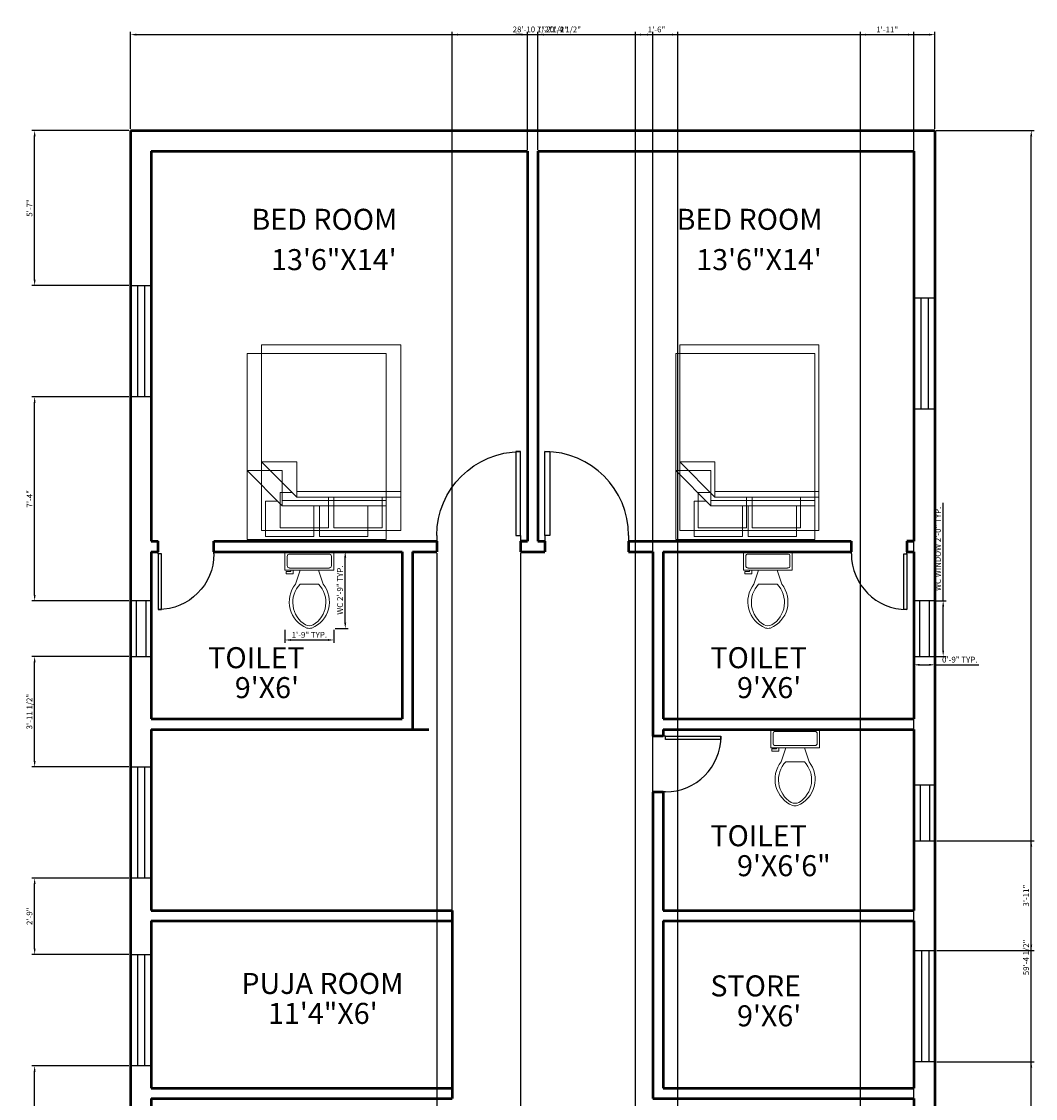
# Model space of a CAD drawing. Units: inches. Extents: x 2691 to 8091, y 3734 to 9067.
# Tile 4 of 5: x 2691 to 3127, y 4181 to 4645. Entities that reach past the tile are written whole.
import ezdxf

# ---------------------------------------------------------------- set-up
doc = ezdxf.new("R2010")
doc.units = ezdxf.units.IN
doc.layers.get('0').update_dxf_attribs({"color": 80})
for name, color, linetype, lineweight in [('A-ANNO-DIMS', 2, 'Continuous', 18), ('A-AREA-IDEN', 7, 'Continuous', 18), ('A-FLOR-FIXT', 9, 'Continuous', 18), ('A-FURN', 8, 'Continuous', 18), ('A-WALL', 50, 'Continuous', 50), ('doors', 10, 'Continuous', 25), ('window', 4, 'Continuous', 25)]:
    doc.layers.add(name, color=color, linetype=linetype, lineweight=lineweight)
doc.styles.get("Standard").update_dxf_attribs({"font": 'arial.ttf'})
doc.dimstyles.new('ISO-25', dxfattribs={"dimtxt": 2.5, "dimasz": 2.5, "dimexe": 1.25, "dimexo": 0.625, "dimtad": 1, "dimdec": 1, "dimlunit": 3, "dimtxsty": 'Standard', "dimcen": 2.5, "dimadec": 0, "dimazin": 0, "dimtfac": 1, "dimtdec": 1, "dimtmove": 0, "dimatfit": 3, "dimfxl": 1, "dimarcsym": 0})

# ---------------------------------------------------------------- blocks, each defined once
blk = doc.blocks.new('Bed - Queen')
for p, q in [((0, -80.00003), (0, 0)), ((0, 0), (59.99999, 0)), ((59.99999, 0), (59.99999, -80.00003)), ((7.99999, -1.2), (28.79998, -1.2)), ((7.99999, -14.4), (7.99999, -1.2)), ((28.79998, -1.2), (28.79998, -14.4)), ((31.19999, -1.2), (51.99999, -1.2)), ((31.19999, -14.4), (31.19999, -1.2)), ((51.99999, -1.2), (51.99999, -16.4)), ((0, -14.4), (44.8, -14.4)), ((44.8, -16.8), (0, -16.8)), ((59.99999, -29.6), (44.8, -14.4)), ((44.8, -14.4), (44.8, -29.6)), ((51.99999, -16.4), (46.79936, -16.4)), ((44.8, -29.6), (59.99999, -29.6)), ((59.99999, -80.00003), (0, -80.00003))]:
    blk.add_line(p, q)
blk = doc.blocks.new('Toilet - top')
for p, q in [((9.5, -6), (9.5, -2)), ((-10, -8.5), (-8, -8.5)), ((-10, -9.5), (-10, -8.5)), ((-8, -8.5), (-8, -8)), ((-7, -8), (-7, -9.5)), ((-4, -8), (-6, -14)), ((4, -8), (6, -14)), ((-7, -9.5), (-10, -9.5)), ((4, -14), (-4, -14))]:
    blk.add_line(p, q)
blk.add_lwpolyline([(10.5, -8), (10.5, 0), (-10.5, 0), (-10.5, -8)], close=True)
for points in [[(-9.5, -2), (-9.5, -6)], [(8.5, -1), (-8.5, -1)], [(-8.5, -7), (8.5, -7)]]:
    blk.add_lwpolyline(points)
for centre, radius, start, end in [((-8.62, -1.88), 0.884, 81.8699, 188.1301), ((8.62, -1.88), 0.884, 351.8699, 98.1301), ((-8.62, -6.12), 0.884, 171.8699, 278.1301), ((8.62, -6.12), 0.884, 261.8699, 8.1301), ((3.52, -21.58), 12.17, 141.4691, 247.9714), ((4.2, -21.82), 11.33, 136.3677, 238.9468), ((-3.52, -21.58), 12.17, 292.0284, 38.5307), ((-4.2, -21.82), 11.33, 301.053, 43.6321), ((0, -27.88), 4, 245.7318, 294.2682), ((0, -29), 4, 254.8605, 285.1395)]:
    blk.add_arc(centre, radius, start, end)
blk = doc.blocks.new('Dining Set - 36 x 72 in')
at = {"layer": 'window'}
for p, q in [((418.4, 887.02), (466.4, 887.02)), ((418.4, 883.92), (466.4, 883.92))]:
    blk.add_line(p, q, dxfattribs=at)
blk.add_lwpolyline([(418.4, 881.14), (418.4, 890.14), (466.4, 890.14), (466.4, 881.14)], close=True, dxfattribs=at)
blk = doc.blocks.new('new block')
at = {"layer": 'window'}
for p, q in [((-15.79, 35.68), (-15.79, 11.68)), ((-11.65, 35.68), (-11.65, 11.68))]:
    blk.add_line(p, q, dxfattribs=at)
blk.add_lwpolyline([(-9.22, 35.68), (-18.22, 35.68), (-18.22, 11.68), (-9.22, 11.68)], close=True, dxfattribs=at)
blk = doc.blocks.new('*U13')
for p, q in [((0, 0), (0, -100)), ((750, 0), (750, -100))]:
    blk.add_line(p, q)
blk.add_lwpolyline([(0, 0), (0, 750), (43.75, 750), (43.75, 0)], close=True)
blk.add_arc((0, 0), 750, 0, 90)
blk = doc.blocks.new('*D23')
at = {"layer": 'A-ANNO-DIMS', "color": 0, "lineweight": -2, "transparency": 16777216}
for p, q in [((3087.56, 4395.22), (3087.56, 4437.39)), ((3084.58, 4395.22), (3088.81, 4395.22)), ((3087.56, 4373.72), (3087.56, 4392.72)), ((3084.58, 4371.22), (3088.81, 4371.22))]:
    blk.add_line(p, q, dxfattribs=at)
at = {"layer": 'A-ANNO-DIMS', "color": 0, "transparency": 16777216}
for points in [[(3087.14, 4392.72), (3087.98, 4392.72), (3087.56, 4395.22)], [(3087.14, 4373.72), (3087.98, 4373.72), (3087.56, 4371.22)]]:
    blk.add_solid(points, dxfattribs=at)
at = {"layer": 'Defpoints', "color": 0, "transparency": 16777216}
for p in [(3083.96, 4395.22), (3087.56, 4395.22), (3083.96, 4371.22)]:
    blk.add_point(p, dxfattribs=at)
at = {"layer": 'A-ANNO-DIMS', "color": 0, "transparency": 16777216, "insert": (3085.64, 4417.56), "char_height": 2.5, "attachment_point": 5, "rotation": 90}
blk.add_mtext('WC WINDOW 2\'-0" TYP.', dxfattribs=at)
blk = doc.blocks.new('*D24')
at = {"layer": 'A-ANNO-DIMS', "color": 0, "lineweight": -2, "transparency": 16777216}
for p, q in [((3074.96, 4370.59), (3074.96, 4366.37)), ((3083.96, 4370.59), (3083.96, 4366.37)), ((3077.46, 4367.62), (3081.46, 4367.62)), ((3083.96, 4367.62), (3102.95, 4367.62))]:
    blk.add_line(p, q, dxfattribs=at)
at = {"layer": 'A-ANNO-DIMS', "color": 0, "transparency": 16777216}
for points in [[(3077.46, 4368.04), (3077.46, 4367.2), (3074.96, 4367.62)], [(3081.46, 4368.04), (3081.46, 4367.2), (3083.96, 4367.62)]]:
    blk.add_solid(points, dxfattribs=at)
at = {"layer": 'Defpoints', "color": 0, "transparency": 16777216}
for p in [(3074.96, 4371.22), (3083.96, 4371.22), (3083.96, 4367.62)]:
    blk.add_point(p, dxfattribs=at)
at = {"layer": 'A-ANNO-DIMS', "color": 0, "transparency": 16777216, "insert": (3094.7, 4369.52), "char_height": 2.5, "attachment_point": 5}
blk.add_mtext('0\'-9" TYP.', dxfattribs=at)
blk = doc.blocks.new('*D31')
at = {"layer": 'A-ANNO-DIMS', "color": 0, "lineweight": -2, "transparency": 16777216}
for p, q in [((2825.66, 4416.32), (2831.24, 4416.32)), ((2829.99, 4385.77), (2829.99, 4413.82)), ((2825.66, 4383.27), (2831.24, 4383.27))]:
    blk.add_line(p, q, dxfattribs=at)
at = {"layer": 'A-ANNO-DIMS', "color": 0, "transparency": 16777216}
for points in [[(2829.57, 4413.82), (2830.41, 4413.82), (2829.99, 4416.32)], [(2829.57, 4385.77), (2830.41, 4385.77), (2829.99, 4383.27)]]:
    blk.add_solid(points, dxfattribs=at)
at = {"layer": 'Defpoints', "color": 0, "transparency": 16777216}
for p in [(2825.03, 4416.32), (2829.99, 4416.32), (2825.03, 4383.27)]:
    blk.add_point(p, dxfattribs=at)
at = {"layer": 'A-ANNO-DIMS', "color": 0, "transparency": 16777216, "insert": (2828.07, 4399.8), "char_height": 2.5, "attachment_point": 5, "rotation": 90}
blk.add_mtext('WC 2\'-9" TYP.', dxfattribs=at)
blk = doc.blocks.new('*D32')
at = {"layer": 'A-ANNO-DIMS', "color": 0, "lineweight": -2, "transparency": 16777216}
for p, q in [((2804.03, 4382.65), (2804.03, 4377.07)), ((2825.03, 4382.65), (2825.03, 4377.07)), ((2806.53, 4378.32), (2822.53, 4378.32))]:
    blk.add_line(p, q, dxfattribs=at)
at = {"layer": 'A-ANNO-DIMS', "color": 0, "transparency": 16777216}
for points in [[(2806.53, 4378.73), (2806.53, 4377.9), (2804.03, 4378.32)], [(2822.53, 4378.73), (2822.53, 4377.9), (2825.03, 4378.32)]]:
    blk.add_solid(points, dxfattribs=at)
at = {"layer": 'Defpoints', "color": 0, "transparency": 16777216}
for p in [(2804.03, 4383.27), (2825.03, 4383.27), (2825.03, 4378.32)]:
    blk.add_point(p, dxfattribs=at)
at = {"layer": 'A-ANNO-DIMS', "color": 0, "transparency": 16777216, "insert": (2814.53, 4380.22), "char_height": 2.5, "attachment_point": 5}
blk.add_mtext('1\'-9" TYP.', dxfattribs=at)
blk = doc.blocks.new('*D45')
at = {"layer": 'A-ANNO-DIMS', "color": 0, "lineweight": -2, "transparency": 16777216}
for p, q in [((2736.83, 4597.82), (2694.95, 4597.82)), ((2696.2, 4533.51), (2696.2, 4595.32)), ((2736.83, 4531.01), (2694.95, 4531.01))]:
    blk.add_line(p, q, dxfattribs=at)
at = {"layer": 'A-ANNO-DIMS', "color": 0, "transparency": 16777216}
for points in [[(2695.79, 4595.32), (2696.62, 4595.32), (2696.2, 4597.82)], [(2695.79, 4533.51), (2696.62, 4533.51), (2696.2, 4531.01)]]:
    blk.add_solid(points, dxfattribs=at)
at = {"layer": 'Defpoints', "color": 0, "transparency": 16777216}
for p in [(2696.2, 4597.82), (2737.46, 4597.82), (2737.46, 4531.01)]:
    blk.add_point(p, dxfattribs=at)
at = {"layer": 'A-ANNO-DIMS', "color": 0, "transparency": 16777216, "insert": (2694.31, 4564.41), "char_height": 2.5, "attachment_point": 5, "rotation": 90}
blk.add_mtext('5\'-7"', dxfattribs=at)
blk = doc.blocks.new('*D46')
at = {"layer": 'A-ANNO-DIMS', "color": 0, "lineweight": -2, "transparency": 16777216}
for p, q in [((2736.83, 4483.01), (2694.95, 4483.01)), ((2696.2, 4397.72), (2696.2, 4480.51)), ((2736.83, 4395.22), (2694.95, 4395.22))]:
    blk.add_line(p, q, dxfattribs=at)
at = {"layer": 'A-ANNO-DIMS', "color": 0, "transparency": 16777216}
for points in [[(2695.79, 4480.51), (2696.62, 4480.51), (2696.2, 4483.01)], [(2695.79, 4397.72), (2696.62, 4397.72), (2696.2, 4395.22)]]:
    blk.add_solid(points, dxfattribs=at)
at = {"layer": 'Defpoints', "color": 0, "transparency": 16777216}
for p in [(2696.2, 4483.01), (2737.46, 4483.01), (2737.45, 4395.22)]:
    blk.add_point(p, dxfattribs=at)
at = {"layer": 'A-ANNO-DIMS', "color": 0, "transparency": 16777216, "insert": (2694.33, 4439.11), "char_height": 2.5, "attachment_point": 5, "rotation": 90}
blk.add_mtext('7\'-4"', dxfattribs=at)
blk = doc.blocks.new('*D47')
at = {"layer": 'A-ANNO-DIMS', "color": 0, "lineweight": -2, "transparency": 16777216}
for p, q in [((2736.83, 4371.22), (2694.95, 4371.22)), ((2696.2, 4326.17), (2696.2, 4368.72)), ((2736.83, 4323.67), (2694.95, 4323.67))]:
    blk.add_line(p, q, dxfattribs=at)
at = {"layer": 'A-ANNO-DIMS', "color": 0, "transparency": 16777216}
for points in [[(2695.79, 4368.72), (2696.62, 4368.72), (2696.2, 4371.22)], [(2695.79, 4326.17), (2696.62, 4326.17), (2696.2, 4323.67)]]:
    blk.add_solid(points, dxfattribs=at)
at = {"layer": 'Defpoints', "color": 0, "transparency": 16777216}
for p in [(2696.2, 4371.22), (2737.45, 4371.22), (2737.46, 4323.67)]:
    blk.add_point(p, dxfattribs=at)
at = {"layer": 'A-ANNO-DIMS', "color": 0, "transparency": 16777216, "insert": (2694.28, 4347.45), "char_height": 2.5, "attachment_point": 5, "rotation": 90}
blk.add_mtext('3\'-11 1/2"', dxfattribs=at)
blk = doc.blocks.new('*D48')
at = {"layer": 'A-ANNO-DIMS', "color": 0, "lineweight": -2, "transparency": 16777216}
for p, q in [((2736.83, 4275.67), (2694.95, 4275.67)), ((2696.2, 4245.39), (2696.2, 4273.17)), ((2736.83, 4242.89), (2694.95, 4242.89))]:
    blk.add_line(p, q, dxfattribs=at)
at = {"layer": 'A-ANNO-DIMS', "color": 0, "transparency": 16777216}
for points in [[(2695.79, 4273.17), (2696.62, 4273.17), (2696.2, 4275.67)], [(2695.79, 4245.39), (2696.62, 4245.39), (2696.2, 4242.89)]]:
    blk.add_solid(points, dxfattribs=at)
at = {"layer": 'Defpoints', "color": 0, "transparency": 16777216}
for p in [(2696.2, 4275.67), (2737.46, 4275.67), (2737.46, 4242.89)]:
    blk.add_point(p, dxfattribs=at)
at = {"layer": 'A-ANNO-DIMS', "color": 0, "transparency": 16777216, "insert": (2694.3, 4259.28), "char_height": 2.5, "attachment_point": 5, "rotation": 90}
blk.add_mtext('2\'-9"', dxfattribs=at)
blk = doc.blocks.new('*D49')
at = {"layer": 'A-ANNO-DIMS', "color": 0, "lineweight": -2, "transparency": 16777216}
for p, q in [((2736.83, 4194.89), (2694.95, 4194.89)), ((2696.2, 4114.35), (2696.2, 4192.39)), ((2736.83, 4111.85), (2694.95, 4111.85))]:
    blk.add_line(p, q, dxfattribs=at)
at = {"layer": 'A-ANNO-DIMS', "color": 0, "transparency": 16777216}
for points in [[(2695.79, 4192.39), (2696.62, 4192.39), (2696.2, 4194.89)], [(2695.79, 4114.35), (2696.62, 4114.35), (2696.2, 4111.85)]]:
    blk.add_solid(points, dxfattribs=at)
at = {"layer": 'Defpoints', "color": 0, "transparency": 16777216}
for p in [(2696.2, 4194.89), (2737.46, 4194.89), (2737.46, 4111.85)]:
    blk.add_point(p, dxfattribs=at)
at = {"layer": 'A-ANNO-DIMS', "color": 0, "transparency": 16777216, "insert": (2694.3, 4153.37), "char_height": 2.5, "attachment_point": 5, "rotation": 90}
blk.add_mtext('6\'-11"', dxfattribs=at)
blk = doc.blocks.new('*D54')
at = {"layer": 'A-ANNO-DIMS', "color": 0, "lineweight": -2, "transparency": 16777216}
for p, q in [((3084.79, 4291.79), (3126.76, 4291.79)), ((3125.51, 4247.07), (3125.51, 4289.29)), ((3084.88, 4244.57), (3126.76, 4244.57))]:
    blk.add_line(p, q, dxfattribs=at)
at = {"layer": 'A-ANNO-DIMS', "color": 0, "transparency": 16777216}
for points in [[(3125.09, 4289.29), (3125.92, 4289.29), (3125.51, 4291.79)], [(3125.09, 4247.07), (3125.92, 4247.07), (3125.51, 4244.57)]]:
    blk.add_solid(points, dxfattribs=at)
at = {"layer": 'Defpoints', "color": 0, "transparency": 16777216}
for p in [(3084.16, 4291.79), (3125.51, 4291.79), (3084.26, 4244.57)]:
    blk.add_point(p, dxfattribs=at)
at = {"layer": 'A-ANNO-DIMS', "color": 0, "transparency": 16777216, "insert": (3123.6, 4268.18), "char_height": 2.5, "attachment_point": 5, "rotation": 90}
blk.add_mtext('3\'-11"', dxfattribs=at)
blk = doc.blocks.new('*D55')
at = {"layer": 'A-ANNO-DIMS', "color": 0, "lineweight": -2, "transparency": 16777216}
for p, q in [((3084.88, 4196.57), (3126.76, 4196.57)), ((3125.51, 4126.91), (3125.51, 4194.07)), ((3084.58, 4124.41), (3126.76, 4124.41))]:
    blk.add_line(p, q, dxfattribs=at)
at = {"layer": 'A-ANNO-DIMS', "color": 0, "transparency": 16777216}
for points in [[(3125.09, 4194.07), (3125.92, 4194.07), (3125.51, 4196.57)], [(3125.09, 4126.91), (3125.92, 4126.91), (3125.51, 4124.41)]]:
    blk.add_solid(points, dxfattribs=at)
at = {"layer": 'Defpoints', "color": 0, "transparency": 16777216}
for p in [(3084.26, 4196.57), (3125.51, 4196.57), (3083.96, 4124.41)]:
    blk.add_point(p, dxfattribs=at)
at = {"layer": 'A-ANNO-DIMS', "color": 0, "transparency": 16777216, "insert": (3123.6, 4160.49), "char_height": 2.5, "attachment_point": 5, "rotation": 90}
blk.add_mtext('6\'-0"', dxfattribs=at)
blk = doc.blocks.new('*D59')
at = {"layer": 'A-ANNO-DIMS', "color": 0, "lineweight": -2, "transparency": 16777216}
for p, q in [((2869.46, 4415.69), (2869.46, 3735.06)), ((2905.46, 4415.69), (2905.46, 3735.06)), ((2871.96, 3736.31), (2902.96, 3736.31))]:
    blk.add_line(p, q, dxfattribs=at)
at = {"layer": 'A-ANNO-DIMS', "color": 0, "transparency": 16777216}
for points in [[(2871.96, 3736.72), (2871.96, 3735.89), (2869.46, 3736.31)], [(2902.96, 3736.72), (2902.96, 3735.89), (2905.46, 3736.31)]]:
    blk.add_solid(points, dxfattribs=at)
at = {"layer": 'Defpoints', "color": 0, "transparency": 16777216}
for p in [(2869.46, 4416.32), (2905.46, 4416.32), (2905.46, 3736.31)]:
    blk.add_point(p, dxfattribs=at)
at = {"layer": 'A-ANNO-DIMS', "color": 0, "transparency": 16777216, "insert": (2887.46, 3738.21), "char_height": 2.5, "attachment_point": 5}
blk.add_mtext('3\'-0"', dxfattribs=at)
blk = doc.blocks.new('*D63')
at = {"layer": 'A-ANNO-DIMS', "color": 0, "lineweight": -2, "transparency": 16777216}
for p, q in [((2954.96, 4031.93), (2954.96, 4640.32)), ((2957.46, 4639.07), (2970.7, 4639.07)), ((2973.2, 4028.91), (2973.2, 4640.32))]:
    blk.add_line(p, q, dxfattribs=at)
at = {"layer": 'A-ANNO-DIMS', "color": 0, "transparency": 16777216}
for points in [[(2957.46, 4639.49), (2957.46, 4638.65), (2954.96, 4639.07)], [(2970.7, 4639.49), (2970.7, 4638.65), (2973.2, 4639.07)]]:
    blk.add_solid(points, dxfattribs=at)
at = {"layer": 'Defpoints', "color": 0, "transparency": 16777216}
for p in [(2973.2, 4639.07), (2954.96, 4031.3), (2973.2, 4028.28)]:
    blk.add_point(p, dxfattribs=at)
at = {"layer": 'A-ANNO-DIMS', "color": 0, "transparency": 16777216, "insert": (2964.08, 4640.97), "char_height": 2.5, "attachment_point": 5}
blk.add_mtext('1\'-6"', dxfattribs=at)
blk = doc.blocks.new('*D64')
at = {"layer": 'A-ANNO-DIMS', "color": 0, "lineweight": -2, "transparency": 16777216}
for p, q in [((3051.89, 4029.3), (3051.89, 4640.32)), ((3054.39, 4639.07), (3072.46, 4639.07)), ((3074.96, 4031.93), (3074.96, 4640.32))]:
    blk.add_line(p, q, dxfattribs=at)
at = {"layer": 'A-ANNO-DIMS', "color": 0, "transparency": 16777216}
for points in [[(3054.39, 4639.49), (3054.39, 4638.65), (3051.89, 4639.07)], [(3072.46, 4639.49), (3072.46, 4638.65), (3074.96, 4639.07)]]:
    blk.add_solid(points, dxfattribs=at)
at = {"layer": 'Defpoints', "color": 0, "transparency": 16777216}
for p in [(3074.96, 4639.07), (3074.96, 4031.3), (3051.89, 4028.68)]:
    blk.add_point(p, dxfattribs=at)
at = {"layer": 'A-ANNO-DIMS', "color": 0, "transparency": 16777216, "insert": (3063.42, 4640.95), "char_height": 2.5, "attachment_point": 5}
blk.add_mtext('1\'-11"', dxfattribs=at)
blk = doc.blocks.new('*D65')
at = {"layer": 'A-ANNO-DIMS', "color": 0, "lineweight": -2, "transparency": 16777216}
for p, q in [((2905.96, 4639.07), (2903.46, 4639.07)), ((2908.46, 4589.44), (2908.46, 4640.32)), ((2908.46, 4639.07), (2912.96, 4639.07)), ((2912.96, 4589.44), (2912.96, 4640.32)), ((2915.46, 4639.07), (2931.68, 4639.07))]:
    blk.add_line(p, q, dxfattribs=at)
at = {"layer": 'A-ANNO-DIMS', "color": 0, "transparency": 16777216}
for points in [[(2905.96, 4639.49), (2905.96, 4638.65), (2908.46, 4639.07)], [(2915.46, 4639.49), (2915.46, 4638.65), (2912.96, 4639.07)]]:
    blk.add_solid(points, dxfattribs=at)
at = {"layer": 'Defpoints', "color": 0, "transparency": 16777216}
for p in [(2912.96, 4639.07), (2908.46, 4588.82), (2912.96, 4588.82)]:
    blk.add_point(p, dxfattribs=at)
at = {"layer": 'A-ANNO-DIMS', "color": 0, "transparency": 16777216, "insert": (2924.82, 4640.99), "char_height": 2.5, "attachment_point": 5}
blk.add_mtext('0\'-4 1/2"', dxfattribs=at)
blk = doc.blocks.new('*D66')
at = {"layer": 'A-ANNO-DIMS', "color": 0, "lineweight": -2, "transparency": 16777216}
for p, q in [((2876.06, 4257.94), (2876.06, 4640.32)), ((2878.56, 4639.07), (2959.96, 4639.07)), ((2962.46, 4257.94), (2962.46, 4640.32))]:
    blk.add_line(p, q, dxfattribs=at)
at = {"layer": 'A-ANNO-DIMS', "color": 0, "transparency": 16777216}
for points in [[(2878.56, 4639.49), (2878.56, 4638.65), (2876.06, 4639.07)], [(2959.96, 4639.49), (2959.96, 4638.65), (2962.46, 4639.07)]]:
    blk.add_solid(points, dxfattribs=at)
at = {"layer": 'Defpoints', "color": 0, "transparency": 16777216}
for p in [(2962.46, 4639.07), (2876.06, 4257.32), (2962.46, 4257.32)]:
    blk.add_point(p, dxfattribs=at)
at = {"layer": 'A-ANNO-DIMS', "color": 0, "transparency": 16777216, "insert": (2919.26, 4640.99), "char_height": 2.5, "attachment_point": 5}
blk.add_mtext('7\'-2 1/2"', dxfattribs=at)
blk = doc.blocks.new('*D67')
at = {"layer": 'A-ANNO-DIMS', "color": 0, "lineweight": -2, "transparency": 16777216}
for p, q in [((2737.46, 4598.44), (2737.46, 4640.32)), ((2739.96, 4639.07), (3081.46, 4639.07)), ((3083.96, 4598.44), (3083.96, 4640.32))]:
    blk.add_line(p, q, dxfattribs=at)
at = {"layer": 'A-ANNO-DIMS', "color": 0, "transparency": 16777216}
for points in [[(2739.96, 4639.49), (2739.96, 4638.65), (2737.46, 4639.07)], [(3081.46, 4639.49), (3081.46, 4638.65), (3083.96, 4639.07)]]:
    blk.add_solid(points, dxfattribs=at)
at = {"layer": 'Defpoints', "color": 0, "transparency": 16777216}
for p in [(3083.96, 4639.07), (2737.46, 4597.82), (3083.96, 4597.82)]:
    blk.add_point(p, dxfattribs=at)
at = {"layer": 'A-ANNO-DIMS', "color": 0, "transparency": 16777216, "insert": (2910.71, 4640.99), "char_height": 2.5, "attachment_point": 5}
blk.add_mtext('28\'-10 1/2"', dxfattribs=at)
blk = doc.blocks.new('*D68')
at = {"layer": 'A-ANNO-DIMS', "color": 0, "lineweight": -2, "transparency": 16777216}
for p, q in [((3084.58, 4597.82), (3126.76, 4597.82)), ((3125.51, 3887.82), (3125.51, 4595.32)), ((3084.58, 3885.32), (3126.76, 3885.32))]:
    blk.add_line(p, q, dxfattribs=at)
at = {"layer": 'A-ANNO-DIMS', "color": 0, "transparency": 16777216}
for points in [[(3125.09, 4595.32), (3125.92, 4595.32), (3125.51, 4597.82)], [(3125.09, 3887.82), (3125.92, 3887.82), (3125.51, 3885.32)]]:
    blk.add_solid(points, dxfattribs=at)
at = {"layer": 'Defpoints', "color": 0, "transparency": 16777216}
for p in [(3083.96, 4597.82), (3125.51, 4597.82), (3083.96, 3885.32)]:
    blk.add_point(p, dxfattribs=at)
at = {"layer": 'A-ANNO-DIMS', "color": 0, "transparency": 16777216, "insert": (3123.59, 4241.57), "char_height": 2.5, "attachment_point": 5, "rotation": 90}
blk.add_mtext('59\'-4 1/2"', dxfattribs=at)

msp = doc.modelspace()

# ---------------------------------------------------------------- linework, layer by layer
at = {"layer": 'A-WALL'}
for p, q in [((2737.46, 4597.82), (2737.46, 3885.32)), ((2737.46, 4597.82), (3083.96, 4597.82)), ((3083.96, 4597.82), (3083.96, 3885.32)), ((2746.46, 4588.82), (2746.46, 4420.82)), ((2746.46, 4588.82), (2908.46, 4588.82)), ((2908.46, 4588.82), (2908.46, 4420.82)), ((2912.96, 4588.82), (2912.96, 4420.82)), ((2912.96, 4588.82), (3074.96, 4588.82)), ((3074.96, 4588.82), (3074.96, 4420.82)), ((2746.46, 4420.82), (2749.46, 4420.82)), ((2746.46, 4416.32), (2749.46, 4416.32)), ((2746.46, 4416.32), (2746.46, 4344.32)), ((2746.46, 4416.32), (2749.46, 4416.32)), ((2749.46, 4416.32), (2749.46, 4420.82)), ((2773.46, 4416.32), (2773.46, 4420.82)), ((2773.46, 4420.82), (2869.46, 4420.82)), ((2773.46, 4416.32), (2854.46, 4416.32)), ((2854.46, 4416.32), (2854.46, 4344.32)), ((2858.96, 4416.32), (2858.96, 4339.82)), ((2858.96, 4416.32), (2869.46, 4416.32)), ((2869.46, 4420.82), (2869.46, 4416.32)), ((2908.46, 4420.82), (2905.46, 4420.82)), ((2905.46, 4420.82), (2905.46, 4416.32)), ((2905.46, 4420.82), (2908.46, 4420.82)), ((2905.46, 4416.32), (2915.96, 4416.32)), ((2912.96, 4420.82), (2915.96, 4420.82)), ((2915.96, 4420.82), (2915.96, 4416.32)), ((2951.96, 4420.82), (2951.96, 4416.32)), ((2951.96, 4420.82), (3047.96, 4420.82)), ((2951.96, 4416.32), (2962.46, 4416.32)), ((2962.46, 4416.32), (2962.46, 4336.82)), ((2966.96, 4416.32), (2966.96, 4344.32)), ((2966.96, 4416.32), (3047.96, 4416.32)), ((3047.96, 4420.82), (3047.96, 4416.32)), ((3074.96, 4420.82), (3071.96, 4420.82)), ((3071.96, 4420.82), (3071.96, 4416.32)), ((3071.96, 4420.82), (3074.96, 4420.82)), ((3071.96, 4416.32), (3074.96, 4416.32)), ((3074.96, 4416.32), (3074.96, 4344.32)), ((2746.46, 4344.32), (2854.46, 4344.32)), ((2966.96, 4344.32), (3074.96, 4344.32)), ((2746.46, 4339.82), (2866.06, 4339.82)), ((2746.46, 4339.82), (2746.46, 4261.82)), ((2966.96, 4339.82), (3074.96, 4339.82)), ((2966.96, 4339.82), (2966.96, 4336.82)), ((2966.96, 4339.82), (2966.96, 4336.82)), ((3074.96, 4339.82), (3074.96, 4261.82)), ((2966.96, 4336.82), (2962.46, 4336.82)), ((2966.96, 4312.82), (2962.46, 4312.82)), ((2962.46, 4312.82), (2962.46, 4257.32)), ((2966.96, 4312.82), (2966.96, 4261.82)), ((2746.46, 4261.82), (2876.06, 4261.82)), ((2876.06, 4261.82), (2876.06, 4180.82)), ((2966.96, 4261.82), (3074.96, 4261.82)), ((2746.46, 4257.32), (2876.06, 4257.32)), ((2746.46, 4257.32), (2746.46, 4185.32)), ((2962.46, 4257.32), (2962.46, 4180.82)), ((2966.96, 4257.32), (2966.96, 4185.32)), ((2966.96, 4257.32), (3074.96, 4257.32)), ((3074.96, 4257.32), (3074.96, 4185.32)), ((2746.46, 4185.32), (2876.06, 4185.32)), ((2966.96, 4185.32), (3074.96, 4185.32)), ((2746.46, 4180.82), (2876.06, 4180.82)), ((2746.46, 4180.82), (2746.46, 4012.82)), ((2962.46, 4180.82), (3074.96, 4180.82)), ((3074.96, 4180.82), (3074.96, 4012.82))]:
    msp.add_line(p, q, dxfattribs=at)

# ---------------------------------------------------------------- block references
at = {"layer": 'A-FLOR-FIXT'}
for p in [(2814.53, 4416.32), (3012.07, 4416.32), (3023.77, 4339.87)]:
    msp.add_blockref('Toilet - top', p, dxfattribs=at)
at = {"layer": 'A-FURN', "rotation": 180}
for p in [(2853.92, 4425.48), (3034.06, 4425.48), (2847.68, 4421.66), (3032.34, 4421.66)]:
    msp.add_blockref('Bed - Queen', p, dxfattribs=at)
at = {"layer": 'doors', "yscale": 0.0481264944431729, "zscale": 0.0481264944431729}
for p, xscale in [((2905.55, 4423.38), -0.0481264944431729), ((2915.96, 4423.38), 0.0481264944431729)]:
    msp.add_blockref('*U13', p, dxfattribs=dict(at, xscale=xscale))
at = {"layer": 'doors', "yscale": 0.0319307598213287, "zscale": 0.0319307598213287}
for p, xscale, rotation in [((2749.46, 4415.38), -0.0319307598213287, 180), ((3071.96, 4415.38), 0.0319307598213287, 179.9999999999875), ((2967.9, 4336.82), 0.0319307598213287, 269.9999999999875)]:
    msp.add_blockref('*U13', p, dxfattribs=dict(at, xscale=xscale, rotation=rotation))
at = {"layer": 'window', "rotation": 90}
for p in [(3627.6, 4064.6), (3965.1, 4059.31), (3627.6, 3857.27), (3627.6, 3776.49), (3965.39, 3778.17)]:
    msp.add_blockref('Dining Set - 36 x 72 in', p, dxfattribs=at)
at = {"layer": 'window'}
for p in [(2755.68, 4359.54), (3093.18, 4359.54), (3093.39, 4280.11)]:
    msp.add_blockref('new block', p, dxfattribs=at)

# ---------------------------------------------------------------- texts
at = {"layer": 'A-AREA-IDEN'}
for s, p in [('BED ROOM', (2789.58, 4554.99)), ('BED ROOM', (2972.74, 4554.99)), ('13\'6"X14\'', (2798.05, 4537.63)), ('13\'6"X14\'', (2981.21, 4537.63)), ('TOILET', (2770.97, 4366.16)), ('TOILET', (2987.29, 4366.16)), ("9'X6'", (2782.44, 4353.26)), ("9'X6'", (2998.76, 4353.26)), ('TOILET', (2987.29, 4289.46)), ('9\'X6\'6"', (2998.76, 4276.56)), ('PUJA ROOM', (2785.26, 4225.84)), ('STORE', (2987.29, 4224.78)), ('11\'4"X6\'', (2796.73, 4212.94)), ("9'X6'", (2998.76, 4211.88))]:
    msp.add_text(s, height=9.054, dxfattribs=at).set_placement(p)

# ---------------------------------------------------------------- dimensions: what is measured, and where the dimension line sits
at = {"layer": 'A-ANNO-DIMS'}
for base, p1, p2, picture, middle in [((3083.96, 4639.07), (2737.46, 4597.82), (3083.96, 4597.82), '*D67', (2910.71, 4640.99)), ((2962.46, 4639.07), (2876.06, 4257.32), (2962.46, 4257.32), '*D66', (2919.26, 4640.99)), ((2912.96, 4639.07), (2908.46, 4588.82), (2912.96, 4588.82), '*D65', (2924.82, 4640.99)), ((2973.2, 4639.07), (2954.96, 4031.3), (2973.2, 4028.28), '*D63', (2964.08, 4640.97)), ((3074.96, 4639.07), (3051.89, 4028.68), (3074.96, 4031.3), '*D64', (3063.42, 4640.95)), ((2905.46, 3736.31), (2869.46, 4416.32), (2905.46, 4416.32), '*D59', (2887.46, 3738.21))]:
    dim = msp.add_linear_dim(base=base, p1=p1, p2=p2, dimstyle='ISO-25', override={"dimdec": 1, "dimlfac": 1, "dimrnd": 0, "dimzin": 1, "dimdsep": 46, "dimlunit": 4, "dimfrac": 2}, dxfattribs=at)
    dim.commit()
    dim.dimension.update_dxf_attribs({"geometry": picture, "text_midpoint": middle})
for base, p1, p2, picture, middle in [((2696.2, 4597.82), (2737.46, 4531.01), (2737.46, 4597.82), '*D45', (2694.31, 4564.41)), ((3125.51, 4597.82), (3083.96, 3885.32), (3083.96, 4597.82), '*D68', (3123.59, 4241.57)), ((2696.2, 4483.01), (2737.45, 4395.22), (2737.46, 4483.01), '*D46', (2694.33, 4439.11)), ((2696.2027, 4371.2183), (2737.4596, 4323.6745), (2737.4527, 4371.2183), '*D47', (2694.2843, 4347.4464)), ((3125.51, 4291.79), (3084.26, 4244.57), (3084.16, 4291.79), '*D54', (3123.6, 4268.18)), ((2696.2, 4275.67), (2737.46, 4242.89), (2737.46, 4275.67), '*D48', (2694.3, 4259.28)), ((2696.2, 4194.89), (2737.46, 4111.85), (2737.46, 4194.89), '*D49', (2694.3, 4153.37)), ((3125.51, 4196.57), (3083.96, 4124.41), (3084.26, 4196.57), '*D55', (3123.6, 4160.49))]:
    dim = msp.add_linear_dim(base=base, p1=p1, p2=p2, angle=90, dimstyle='ISO-25', override={"dimdec": 1, "dimlfac": 1, "dimrnd": 0, "dimzin": 1, "dimdsep": 46, "dimlunit": 4, "dimfrac": 2}, dxfattribs=at)
    dim.commit()
    dim.dimension.update_dxf_attribs({"geometry": picture, "text_midpoint": middle})
for base, p1, p2, text, picture, middle in [((3087.56, 4395.22), (3083.96, 4371.22), (3083.96, 4395.22), 'WC WINDOW <> TYP.', '*D23', (3085.64, 4417.56)), ((2829.9902, 4416.3188), (2825.0333, 4383.2726), (2825.0333, 4416.3188), 'WC <> TYP.', '*D31', (2828.0726, 4399.7957))]:
    dim = msp.add_linear_dim(base=base, p1=p1, p2=p2, angle=90, text=text, dimstyle='ISO-25', override={"dimdec": 1, "dimlfac": 1, "dimrnd": 0, "dimzin": 1, "dimdsep": 46, "dimlunit": 4, "dimfrac": 2}, dxfattribs=at)
    dim.commit()
    dim.dimension.update_dxf_attribs({"geometry": picture, "text_midpoint": middle})
for base, p1, p2, picture, middle in [((2825.03, 4378.32), (2804.03, 4383.27), (2825.03, 4383.27), '*D32', (2814.53, 4380.22)), ((3083.96, 4367.62), (3074.96, 4371.22), (3083.96, 4371.22), '*D24', (3094.7, 4369.52))]:
    dim = msp.add_linear_dim(base=base, p1=p1, p2=p2, text='<> TYP.', dimstyle='ISO-25', override={"dimdec": 1, "dimlfac": 1, "dimrnd": 0, "dimzin": 1, "dimdsep": 46, "dimlunit": 4, "dimfrac": 2}, dxfattribs=at)
    dim.commit()
    dim.dimension.update_dxf_attribs({"geometry": picture, "text_midpoint": middle})

doc.saveas('drawing.dxf')
